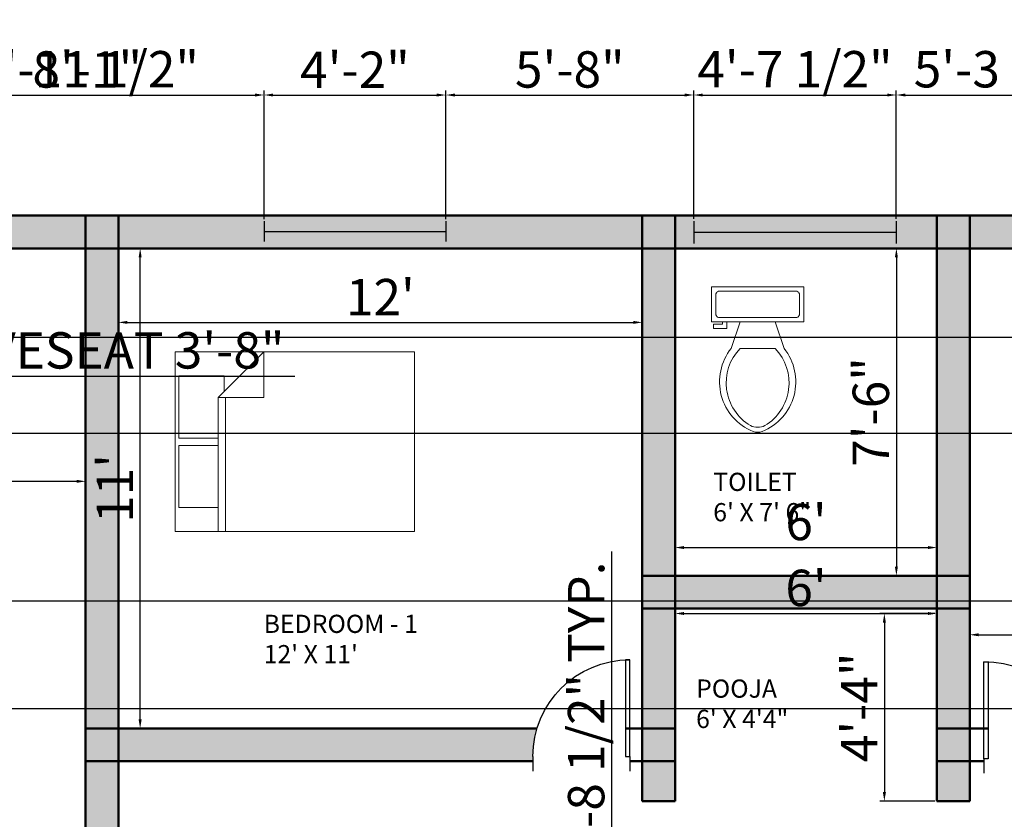
# Model space of a CAD drawing. Units: millimetres. Extents: x 2208 to 3043, y 878 to 1386.
# Tile 3 of 4: x 2479 to 2749, y 1166 to 1386. Entities that reach past the tile are written whole.
import ezdxf

# ---------------------------------------------------------------- set-up
doc = ezdxf.new("R2010")
doc.units = ezdxf.units.MM
for name, color, linetype, lineweight in [('A-ANNO-DIMS', 50, 'Continuous', 13), ('A-AREA-IDEN', 90, 'Continuous', 25), ('A-FLOR-FIXT', 140, 'Continuous', 18), ('A-WALL-PATT', 6, 'Continuous', 13), ('doors', 30, 'Continuous', 25), ('furniture', 140, 'Continuous', 18), ('walls', 200, 'Continuous', 50), ('windows', 10, 'Continuous', 25)]:
    doc.layers.add(name, color=color, linetype=linetype, lineweight=lineweight)
doc.styles.get("Standard").update_dxf_attribs({"font": 'arial.ttf'})
doc.dimstyles.new('ISO-25', dxfattribs={"dimtxt": 10, "dimasz": 2.5, "dimexe": 1.25, "dimexo": 0.625, "dimtad": 1, "dimdec": 0, "dimlunit": 3, "dimtxsty": 'Standard', "dimcen": 2.5, "dimadec": 0, "dimazin": 0, "dimtfac": 1, "dimtdec": 0, "dimtmove": 0, "dimatfit": 3, "dimfxl": 1, "dimarcsym": 0})

# ---------------------------------------------------------------- blocks, each defined once
blk = doc.blocks.new('*U2')
for p, q in [((0, 0), (0, -6)), ((40, 0), (40, -6))]:
    blk.add_line(p, q)
blk.add_lwpolyline([(0, 0), (0, 40), (1.75, 40), (1.75, 0)], close=True)
blk.add_arc((0, 0), 40, 0, 90)
blk = doc.blocks.new('*U4')
for p, q in [((0, 4), (0, 0)), ((36, 4), (36, 0)), ((0, 2), (36, 2))]:
    blk.add_line(p, q)
blk = doc.blocks.new('*U5')
for p, q in [((0, 4), (0, 0)), ((36, 4), (36, 0)), ((0, 2), (36, 2))]:
    blk.add_line(p, q)
blk = doc.blocks.new('Bed - Queen')
for p, q in [((0, -80.00003), (0, 0)), ((0, 0), (59.99999, 0)), ((59.99999, 0), (59.99999, -80.00003)), ((7.99999, -1.2), (28.79998, -1.2)), ((7.99999, -14.4), (7.99999, -1.2)), ((28.79998, -1.2), (28.79998, -14.4)), ((31.19999, -1.2), (51.99999, -1.2)), ((31.19999, -14.4), (31.19999, -1.2)), ((51.99999, -1.2), (51.99999, -16.4)), ((0, -14.4), (44.8, -14.4)), ((59.99999, -29.6), (44.8, -14.4)), ((44.8, -14.4), (44.8, -29.6)), ((51.99999, -16.4), (46.79936, -16.4)), ((44.8, -16.8), (0, -16.8)), ((44.8, -29.6), (59.99999, -29.6)), ((59.99999, -80.00003), (0, -80.00003))]:
    blk.add_line(p, q)
blk = doc.blocks.new('Toilet - top')
for p, q in [((9.5, -6), (9.5, -2)), ((-10, -8.5), (-8, -8.5)), ((-10, -9.5), (-10, -8.5)), ((-8, -8.5), (-8, -8)), ((-7, -8), (-7, -9.5)), ((-4, -8), (-6, -14)), ((4, -8), (6, -14)), ((-7, -9.5), (-10, -9.5)), ((4, -14), (-4, -14))]:
    blk.add_line(p, q)
blk.add_lwpolyline([(10.5, -8), (10.5, 0), (-10.5, 0), (-10.5, -8)], close=True)
for points in [[(-9.5, -2), (-9.5, -6)], [(8.5, -1), (-8.5, -1)], [(-8.5, -7), (8.5, -7)]]:
    blk.add_lwpolyline(points)
for centre, radius, start, end in [((-8.62, -1.88), 0.884, 81.8699, 188.1301), ((8.62, -1.88), 0.884, 351.8699, 98.1301), ((-8.62, -6.12), 0.884, 171.8699, 278.1301), ((8.62, -6.12), 0.884, 261.8699, 8.1301), ((3.52, -21.58), 12.17, 141.4691, 247.9714), ((4.2, -21.82), 11.33, 136.3677, 238.9468), ((-3.52, -21.58), 12.17, 292.0284, 38.5307), ((-4.2, -21.82), 11.33, 301.053, 43.6321), ((0, -27.88), 4, 245.7318, 294.2682), ((0, -29), 4, 254.8605, 285.1395)]:
    blk.add_arc(centre, radius, start, end)
blk = doc.blocks.new('*D13')
at = {"layer": 'A-ANNO-DIMS', "color": 0, "lineweight": -2, "transparency": 16777216}
for p, q in [((2505.98, 1310.26), (2505.98, 1301.83)), ((2649.98, 1310.26), (2649.98, 1301.83)), ((2508.48, 1303.08), (2647.48, 1303.08))]:
    blk.add_line(p, q, dxfattribs=at)
at = {"layer": 'A-ANNO-DIMS', "color": 0, "transparency": 16777216}
for points in [[(2508.48, 1303.5), (2508.48, 1302.67), (2505.98, 1303.08)], [(2647.48, 1303.5), (2647.48, 1302.67), (2649.98, 1303.08)]]:
    blk.add_solid(points, dxfattribs=at)
at = {"layer": 'Defpoints', "color": 0, "transparency": 16777216}
for p in [(2505.98, 1310.88), (2649.98, 1310.88), (2649.98, 1303.08)]:
    blk.add_point(p, dxfattribs=at)
at = {"layer": 'A-ANNO-DIMS', "color": 0, "transparency": 16777216, "insert": (2577.98, 1308.73), "char_height": 10, "attachment_point": 5}
blk.add_mtext("12'", dxfattribs=at)
blk = doc.blocks.new('*D14')
at = {"layer": 'A-ANNO-DIMS', "color": 0, "lineweight": -2, "transparency": 16777216}
for p, q in [((2514.03, 1323.44), (2510.71, 1323.44)), ((2511.96, 1193.94), (2511.96, 1320.94)), ((2514.03, 1191.44), (2510.71, 1191.44))]:
    blk.add_line(p, q, dxfattribs=at)
at = {"layer": 'A-ANNO-DIMS', "color": 0, "transparency": 16777216}
for points in [[(2511.54, 1320.94), (2512.37, 1320.94), (2511.96, 1323.44)], [(2511.54, 1193.94), (2512.37, 1193.94), (2511.96, 1191.44)]]:
    blk.add_solid(points, dxfattribs=at)
at = {"layer": 'Defpoints', "color": 0, "transparency": 16777216}
for p in [(2511.96, 1323.44), (2514.65, 1323.44), (2514.65, 1191.44)]:
    blk.add_point(p, dxfattribs=at)
at = {"layer": 'A-ANNO-DIMS', "color": 0, "transparency": 16777216, "insert": (2506.31, 1257.44), "char_height": 10, "attachment_point": 5, "rotation": 90}
blk.add_mtext("11'", dxfattribs=at)
blk = doc.blocks.new('*D15')
at = {"layer": 'A-ANNO-DIMS', "color": 0, "lineweight": -2, "transparency": 16777216}
for p, q in [((2352.98, 1251.32), (2352.98, 1260.64)), ((2355.48, 1259.39), (2494.48, 1259.39)), ((2496.98, 1251.32), (2496.98, 1260.64))]:
    blk.add_line(p, q, dxfattribs=at)
at = {"layer": 'A-ANNO-DIMS', "color": 0, "transparency": 16777216}
for points in [[(2355.48, 1259.81), (2355.48, 1258.97), (2352.98, 1259.39)], [(2494.48, 1259.81), (2494.48, 1258.97), (2496.98, 1259.39)]]:
    blk.add_solid(points, dxfattribs=at)
at = {"layer": 'Defpoints', "color": 0, "transparency": 16777216}
for p in [(2496.98, 1259.39), (2352.98, 1250.7), (2496.98, 1250.7)]:
    blk.add_point(p, dxfattribs=at)
at = {"layer": 'A-ANNO-DIMS', "color": 0, "transparency": 16777216, "insert": (2424.98, 1265.03), "char_height": 10, "attachment_point": 5}
blk.add_mtext("12'", dxfattribs=at)
blk = doc.blocks.new('*D17')
at = {"layer": 'A-ANNO-DIMS', "color": 0, "lineweight": -2, "transparency": 16777216}
for p, q in [((2658.98, 1251.31), (2658.98, 1239.93)), ((2730.98, 1251.31), (2730.98, 1239.93)), ((2661.48, 1241.18), (2728.48, 1241.18))]:
    blk.add_line(p, q, dxfattribs=at)
at = {"layer": 'A-ANNO-DIMS', "color": 0, "transparency": 16777216}
for points in [[(2661.48, 1241.6), (2661.48, 1240.77), (2658.98, 1241.18)], [(2728.48, 1241.6), (2728.48, 1240.77), (2730.98, 1241.18)]]:
    blk.add_solid(points, dxfattribs=at)
at = {"layer": 'Defpoints', "color": 0, "transparency": 16777216}
for p in [(2658.98, 1251.94), (2730.98, 1251.94), (2730.98, 1241.18)]:
    blk.add_point(p, dxfattribs=at)
at = {"layer": 'A-ANNO-DIMS', "color": 0, "transparency": 16777216, "insert": (2694.98, 1246.91), "char_height": 10, "attachment_point": 5}
blk.add_mtext("6'", dxfattribs=at)
blk = doc.blocks.new('*D18')
at = {"layer": 'A-ANNO-DIMS', "color": 0, "lineweight": -2, "transparency": 16777216}
for p, q in [((2709.59, 1323.44), (2721.07, 1323.44)), ((2719.82, 1320.94), (2719.82, 1235.94)), ((2709.59, 1233.44), (2721.07, 1233.44))]:
    blk.add_line(p, q, dxfattribs=at)
at = {"layer": 'A-ANNO-DIMS', "color": 0, "transparency": 16777216}
for points in [[(2719.41, 1320.94), (2720.24, 1320.94), (2719.82, 1323.44)], [(2719.41, 1235.94), (2720.24, 1235.94), (2719.82, 1233.44)]]:
    blk.add_solid(points, dxfattribs=at)
at = {"layer": 'Defpoints', "color": 0, "transparency": 16777216}
for p in [(2708.97, 1323.44), (2708.97, 1233.44), (2719.82, 1233.44)]:
    blk.add_point(p, dxfattribs=at)
at = {"layer": 'A-ANNO-DIMS', "color": 0, "transparency": 16777216, "insert": (2714.09, 1278.44), "char_height": 10, "attachment_point": 5, "rotation": 90}
blk.add_mtext('7\'-6"', dxfattribs=at)
blk = doc.blocks.new('*D19')
at = {"layer": 'A-ANNO-DIMS', "color": 0, "lineweight": -2, "transparency": 16777216}
for p, q in [((2739.98, 1223.81), (2739.98, 1215.95)), ((2913.98, 1223.81), (2913.98, 1215.95)), ((2742.48, 1217.2), (2911.48, 1217.2))]:
    blk.add_line(p, q, dxfattribs=at)
at = {"layer": 'A-ANNO-DIMS', "color": 0, "transparency": 16777216}
for points in [[(2742.48, 1217.62), (2742.48, 1216.78), (2739.98, 1217.2)], [(2911.48, 1217.62), (2911.48, 1216.78), (2913.98, 1217.2)]]:
    blk.add_solid(points, dxfattribs=at)
at = {"layer": 'Defpoints', "color": 0, "transparency": 16777216}
for p in [(2739.98, 1224.44), (2913.98, 1224.44), (2913.98, 1217.2)]:
    blk.add_point(p, dxfattribs=at)
at = {"layer": 'A-ANNO-DIMS', "color": 0, "transparency": 16777216, "insert": (2826.98, 1222.93), "char_height": 10, "attachment_point": 5}
blk.add_mtext('14\'-6"', dxfattribs=at)
blk = doc.blocks.new('*D31')
at = {"layer": 'A-ANNO-DIMS', "color": 0, "lineweight": -2, "transparency": 16777216}
for p, q in [((2658.98, 1216.36), (2658.98, 1224.31)), ((2730.98, 1216.36), (2730.98, 1224.31)), ((2661.48, 1223.06), (2728.48, 1223.06))]:
    blk.add_line(p, q, dxfattribs=at)
at = {"layer": 'A-ANNO-DIMS', "color": 0, "transparency": 16777216}
for points in [[(2661.48, 1223.47), (2661.48, 1222.64), (2658.98, 1223.06)], [(2728.48, 1223.47), (2728.48, 1222.64), (2730.98, 1223.06)]]:
    blk.add_solid(points, dxfattribs=at)
at = {"layer": 'Defpoints', "color": 0, "transparency": 16777216}
for p in [(2730.98, 1223.06), (2658.98, 1215.74), (2730.98, 1215.74)]:
    blk.add_point(p, dxfattribs=at)
at = {"layer": 'A-ANNO-DIMS', "color": 0, "transparency": 16777216, "insert": (2694.98, 1228.79), "char_height": 10, "attachment_point": 5}
blk.add_mtext("6'", dxfattribs=at)
blk = doc.blocks.new('*D32')
at = {"layer": 'A-ANNO-DIMS', "color": 0, "lineweight": -2, "transparency": 16777216}
for p, q in [((2730.36, 1223.06), (2715.27, 1223.06)), ((2716.52, 1220.56), (2716.52, 1173.94)), ((2730.36, 1171.44), (2715.27, 1171.44))]:
    blk.add_line(p, q, dxfattribs=at)
at = {"layer": 'A-ANNO-DIMS', "color": 0, "transparency": 16777216}
for points in [[(2716.11, 1220.56), (2716.94, 1220.56), (2716.52, 1223.06)], [(2716.11, 1173.94), (2716.94, 1173.94), (2716.52, 1171.44)]]:
    blk.add_solid(points, dxfattribs=at)
at = {"layer": 'Defpoints', "color": 0, "transparency": 16777216}
for p in [(2730.98, 1223.06), (2716.52, 1171.44), (2730.98, 1171.44)]:
    blk.add_point(p, dxfattribs=at)
at = {"layer": 'A-ANNO-DIMS', "color": 0, "transparency": 16777216, "insert": (2710.9, 1197.25), "char_height": 10, "attachment_point": 5, "rotation": 90}
blk.add_mtext('4\'-4"', dxfattribs=at)
blk = doc.blocks.new('*D34')
at = {"layer": 'A-ANNO-DIMS', "color": 0, "lineweight": -2, "transparency": 16777216}
for p, q in [((2641.64, 1104.85), (2641.64, 1240.09)), ((2642.27, 1104.85), (2640.39, 1104.85)), ((2641.64, 1099.01), (2641.64, 1102.35)), ((2642.27, 1096.51), (2640.39, 1096.51))]:
    blk.add_line(p, q, dxfattribs=at)
at = {"layer": 'A-ANNO-DIMS', "color": 0, "transparency": 16777216}
for points in [[(2641.22, 1102.35), (2642.06, 1102.35), (2641.64, 1104.85)], [(2641.22, 1099.01), (2642.06, 1099.01), (2641.64, 1096.51)]]:
    blk.add_solid(points, dxfattribs=at)
at = {"layer": 'Defpoints', "color": 0, "transparency": 16777216}
for p in [(2641.64, 1104.85), (2642.89, 1104.85), (2642.89, 1096.51)]:
    blk.add_point(p, dxfattribs=at)
at = {"layer": 'A-ANNO-DIMS', "color": 0, "transparency": 16777216, "insert": (2635.84, 1173.72), "char_height": 10, "attachment_point": 5, "rotation": 90}
blk.add_mtext('CHAIR 0\'-8 1/2" TYP.', dxfattribs=at)
blk = doc.blocks.new('*D44')
at = {"layer": 'A-ANNO-DIMS', "color": 0, "lineweight": -2, "transparency": 16777216}
for p, q in [((2402.99, 1294.26), (2402.99, 1287.04)), ((2446.98, 1294.26), (2446.98, 1287.04)), ((2405.49, 1288.29), (2444.48, 1288.29)), ((2446.98, 1288.29), (2554.51, 1288.29))]:
    blk.add_line(p, q, dxfattribs=at)
at = {"layer": 'A-ANNO-DIMS', "color": 0, "transparency": 16777216}
for points in [[(2405.49, 1288.7), (2405.49, 1287.87), (2402.99, 1288.29)], [(2444.48, 1288.7), (2444.48, 1287.87), (2446.98, 1288.29)]]:
    blk.add_solid(points, dxfattribs=at)
at = {"layer": 'Defpoints', "color": 0, "transparency": 16777216}
for p in [(2402.99, 1294.89), (2446.98, 1294.89), (2446.98, 1288.29)]:
    blk.add_point(p, dxfattribs=at)
at = {"layer": 'A-ANNO-DIMS', "color": 0, "transparency": 16777216, "insert": (2502, 1294.09), "char_height": 10, "attachment_point": 5}
blk.add_mtext('LOVESEAT 3\'-8"', dxfattribs=at)
blk = doc.blocks.new('*D47')
at = {"layer": 'A-ANNO-DIMS', "color": 0, "lineweight": -2, "transparency": 16777216}
for p, q in [((2343.36, 1332.44), (2309.12, 1332.44)), ((2310.37, 1329.94), (2310.37, 923.22)), ((2589.36, 920.72), (2309.12, 920.72))]:
    blk.add_line(p, q, dxfattribs=at)
at = {"layer": 'A-ANNO-DIMS', "color": 0, "transparency": 16777216}
for points in [[(2309.95, 1329.94), (2310.79, 1329.94), (2310.37, 1332.44)], [(2309.95, 923.22), (2310.79, 923.22), (2310.37, 920.72)]]:
    blk.add_solid(points, dxfattribs=at)
at = {"layer": 'Defpoints', "color": 0, "transparency": 16777216}
for p in [(2343.98, 1332.44), (2310.37, 920.72), (2589.98, 920.72)]:
    blk.add_point(p, dxfattribs=at)
at = {"layer": 'A-ANNO-DIMS', "color": 0, "transparency": 16777216, "insert": (2304.57, 1126.58), "char_height": 10, "attachment_point": 5, "rotation": 90}
blk.add_mtext('34\'-3 1/2"', dxfattribs=at)
blk = doc.blocks.new('*D51')
at = {"layer": 'A-ANNO-DIMS', "color": 0, "lineweight": -2, "transparency": 16777216}
for p, q in [((2344.15, 1299.03), (3035.56, 1299.03)), ((3034.31, 1296.53), (3034.31, 1275.14)), ((2344.61, 1272.64), (3035.56, 1272.64)), ((3034.31, 1272.64), (3034.31, 1218.83))]:
    blk.add_line(p, q, dxfattribs=at)
at = {"layer": 'A-ANNO-DIMS', "color": 0, "transparency": 16777216}
for points in [[(3033.9, 1296.53), (3034.73, 1296.53), (3034.31, 1299.03)], [(3033.9, 1275.14), (3034.73, 1275.14), (3034.31, 1272.64)]]:
    blk.add_solid(points, dxfattribs=at)
at = {"layer": 'Defpoints', "color": 0, "transparency": 16777216}
for p in [(2343.52, 1299.03), (2343.98, 1272.64), (3034.31, 1272.64)]:
    blk.add_point(p, dxfattribs=at)
at = {"layer": 'A-ANNO-DIMS', "color": 0, "transparency": 16777216, "insert": (3028.52, 1244.49), "char_height": 10, "attachment_point": 5, "rotation": 90}
blk.add_mtext('2\'-2 1/2"', dxfattribs=at)
blk = doc.blocks.new('*D55')
at = {"layer": 'A-ANNO-DIMS', "color": 0, "lineweight": -2, "transparency": 16777216}
for p, q in [((2448.81, 1332.56), (2448.81, 1366.84)), ((2546.02, 1331.5), (2546.02, 1366.84)), ((2451.31, 1365.59), (2543.52, 1365.59))]:
    blk.add_line(p, q, dxfattribs=at)
at = {"layer": 'A-ANNO-DIMS', "color": 0, "transparency": 16777216}
for points in [[(2451.31, 1366), (2451.31, 1365.17), (2448.81, 1365.59)], [(2543.52, 1366), (2543.52, 1365.17), (2546.02, 1365.59)]]:
    blk.add_solid(points, dxfattribs=at)
at = {"layer": 'Defpoints', "color": 0, "transparency": 16777216}
for p in [(2546.02, 1365.59), (2448.81, 1331.94), (2546.02, 1330.88)]:
    blk.add_point(p, dxfattribs=at)
at = {"layer": 'A-ANNO-DIMS', "color": 0, "transparency": 16777216, "insert": (2497.42, 1371.32), "char_height": 10, "attachment_point": 5}
blk.add_mtext('8\'-1"', dxfattribs=at)
blk = doc.blocks.new('*D56')
at = {"layer": 'A-ANNO-DIMS', "color": 0, "lineweight": -2, "transparency": 16777216}
for p, q in [((2546.02, 1331.5), (2546.02, 1366.84)), ((2595.97, 1331.5), (2595.97, 1366.84)), ((2548.52, 1365.59), (2593.47, 1365.59))]:
    blk.add_line(p, q, dxfattribs=at)
at = {"layer": 'A-ANNO-DIMS', "color": 0, "transparency": 16777216}
for points in [[(2548.52, 1366), (2548.52, 1365.17), (2546.02, 1365.59)], [(2593.47, 1366), (2593.47, 1365.17), (2595.97, 1365.59)]]:
    blk.add_solid(points, dxfattribs=at)
at = {"layer": 'Defpoints', "color": 0, "transparency": 16777216}
for p in [(2595.97, 1365.59), (2546.02, 1330.88), (2595.97, 1330.88)]:
    blk.add_point(p, dxfattribs=at)
at = {"layer": 'A-ANNO-DIMS', "color": 0, "transparency": 16777216, "insert": (2571, 1371.23), "char_height": 10, "attachment_point": 5}
blk.add_mtext('4\'-2"', dxfattribs=at)
blk = doc.blocks.new('*D57')
at = {"layer": 'A-ANNO-DIMS', "color": 0, "lineweight": -2, "transparency": 16777216}
for p, q in [((2595.97, 1331.5), (2595.97, 1366.84)), ((2664.12, 1331.57), (2664.12, 1366.84)), ((2598.47, 1365.59), (2661.62, 1365.59))]:
    blk.add_line(p, q, dxfattribs=at)
at = {"layer": 'A-ANNO-DIMS', "color": 0, "transparency": 16777216}
for points in [[(2598.47, 1366), (2598.47, 1365.17), (2595.97, 1365.59)], [(2661.62, 1366), (2661.62, 1365.17), (2664.12, 1365.59)]]:
    blk.add_solid(points, dxfattribs=at)
at = {"layer": 'Defpoints', "color": 0, "transparency": 16777216}
for p in [(2664.12, 1365.59), (2595.97, 1330.88), (2664.12, 1330.94)]:
    blk.add_point(p, dxfattribs=at)
at = {"layer": 'A-ANNO-DIMS', "color": 0, "transparency": 16777216, "insert": (2630.05, 1371.32), "char_height": 10, "attachment_point": 5}
blk.add_mtext('5\'-8"', dxfattribs=at)
blk = doc.blocks.new('*D58')
at = {"layer": 'A-ANNO-DIMS', "color": 0, "lineweight": -2, "transparency": 16777216}
for p, q in [((2664.12, 1331.57), (2664.12, 1366.84)), ((2719.8, 1331.57), (2719.8, 1366.84)), ((2666.62, 1365.59), (2717.3, 1365.59))]:
    blk.add_line(p, q, dxfattribs=at)
at = {"layer": 'A-ANNO-DIMS', "color": 0, "transparency": 16777216}
for points in [[(2666.62, 1366), (2666.62, 1365.17), (2664.12, 1365.59)], [(2717.3, 1366), (2717.3, 1365.17), (2719.8, 1365.59)]]:
    blk.add_solid(points, dxfattribs=at)
at = {"layer": 'Defpoints', "color": 0, "transparency": 16777216}
for p in [(2719.8, 1365.59), (2664.12, 1330.94), (2719.8, 1330.94)]:
    blk.add_point(p, dxfattribs=at)
at = {"layer": 'A-ANNO-DIMS', "color": 0, "transparency": 16777216, "insert": (2691.96, 1371.38), "char_height": 10, "attachment_point": 5}
blk.add_mtext('4\'-7 1/2"', dxfattribs=at)
blk = doc.blocks.new('*D59')
at = {"layer": 'A-ANNO-DIMS', "color": 0, "lineweight": -2, "transparency": 16777216}
for p, q in [((2719.8, 1331.57), (2719.8, 1366.84)), ((2783.08, 1330.66), (2783.08, 1366.84)), ((2722.3, 1365.59), (2780.58, 1365.59))]:
    blk.add_line(p, q, dxfattribs=at)
at = {"layer": 'A-ANNO-DIMS', "color": 0, "transparency": 16777216}
for points in [[(2722.3, 1366), (2722.3, 1365.17), (2719.8, 1365.59)], [(2780.58, 1366), (2780.58, 1365.17), (2783.08, 1365.59)]]:
    blk.add_solid(points, dxfattribs=at)
at = {"layer": 'Defpoints', "color": 0, "transparency": 16777216}
for p in [(2783.08, 1365.59), (2719.8, 1330.94), (2783.08, 1330.03)]:
    blk.add_point(p, dxfattribs=at)
at = {"layer": 'A-ANNO-DIMS', "color": 0, "transparency": 16777216, "insert": (2751.44, 1371.38), "char_height": 10, "attachment_point": 5}
blk.add_mtext('5\'-3 1/2"', dxfattribs=at)
blk = doc.blocks.new('*D63')
at = {"layer": 'A-ANNO-DIMS', "color": 0, "lineweight": -2, "transparency": 16777216}
for p, q in [((2406.08, 1227.17), (2406.08, 1366.84)), ((2465.35, 1227.17), (2465.35, 1366.84)), ((2408.58, 1365.59), (2462.85, 1365.59)), ((2465.35, 1365.59), (2527.15, 1365.59))]:
    blk.add_line(p, q, dxfattribs=at)
at = {"layer": 'A-ANNO-DIMS', "color": 0, "transparency": 16777216}
for points in [[(2408.58, 1366), (2408.58, 1365.17), (2406.08, 1365.59)], [(2462.85, 1366), (2462.85, 1365.17), (2465.35, 1365.59)]]:
    blk.add_solid(points, dxfattribs=at)
at = {"layer": 'Defpoints', "color": 0, "transparency": 16777216}
for p in [(2465.35, 1365.59), (2406.08, 1226.55), (2465.35, 1226.55)]:
    blk.add_point(p, dxfattribs=at)
at = {"layer": 'A-ANNO-DIMS', "color": 0, "transparency": 16777216, "insert": (2497.5, 1371.38), "char_height": 10, "attachment_point": 5}
blk.add_mtext('4\'-11 1/2"', dxfattribs=at)
blk = doc.blocks.new('*D64')
at = {"layer": 'A-ANNO-DIMS', "color": 0, "lineweight": -2, "transparency": 16777216}
for p, q in [((3034.31, 1226.55), (3034.31, 1280.35)), ((2465.97, 1226.55), (3035.56, 1226.55)), ((3034.31, 1199.41), (3034.31, 1224.05)), ((2465.97, 1196.91), (3035.56, 1196.91))]:
    blk.add_line(p, q, dxfattribs=at)
at = {"layer": 'A-ANNO-DIMS', "color": 0, "transparency": 16777216}
for points in [[(3033.9, 1224.05), (3034.73, 1224.05), (3034.31, 1226.55)], [(3033.9, 1199.41), (3034.73, 1199.41), (3034.31, 1196.91)]]:
    blk.add_solid(points, dxfattribs=at)
at = {"layer": 'Defpoints', "color": 0, "transparency": 16777216}
for p in [(2465.35, 1226.55), (3034.31, 1226.55), (2465.35, 1196.91)]:
    blk.add_point(p, dxfattribs=at)
at = {"layer": 'A-ANNO-DIMS', "color": 0, "transparency": 16777216, "insert": (3028.52, 1254.7), "char_height": 10, "attachment_point": 5, "rotation": 90}
blk.add_mtext('2\'-5 1/2"', dxfattribs=at)
blk = doc.blocks.new('*D66')
at = {"layer": 'A-ANNO-DIMS', "color": 0, "lineweight": -2, "transparency": 16777216}
for p, q in [((3034.31, 1140.35), (3034.31, 1201.74)), ((2674.33, 1140.35), (3035.56, 1140.35)), ((3034.31, 1095.26), (3034.31, 1137.85)), ((2673.86, 1092.76), (3035.56, 1092.76))]:
    blk.add_line(p, q, dxfattribs=at)
at = {"layer": 'A-ANNO-DIMS', "color": 0, "transparency": 16777216}
for points in [[(3033.9, 1137.85), (3034.73, 1137.85), (3034.31, 1140.35)], [(3033.9, 1095.26), (3034.73, 1095.26), (3034.31, 1092.76)]]:
    blk.add_solid(points, dxfattribs=at)
at = {"layer": 'Defpoints', "color": 0, "transparency": 16777216}
for p in [(2673.7, 1140.35), (3034.31, 1140.35), (2673.23, 1092.76)]:
    blk.add_point(p, dxfattribs=at)
at = {"layer": 'A-ANNO-DIMS', "color": 0, "transparency": 16777216, "insert": (3028.52, 1172.3), "char_height": 10, "attachment_point": 5, "rotation": 90}
blk.add_mtext('3\'-11 1/2"', dxfattribs=at)

msp = doc.modelspace()

# ---------------------------------------------------------------- hatches: boundary and pattern name
at = {"layer": 'A-WALL-PATT'}
h = msp.add_hatch(color=256, dxfattribs=at)
h.dxf.hatch_style = 1
h.paths.add_polyline_path([(2352.98, 1273, -0.051847), (2347.51, 1272.43), (2343.98, 1272.43), (2343.98, 1137.44), (2352.98, 1137.44)])
h.paths.add_polyline_path([(2352.98, 1323.44), (2343.98, 1323.44), (2343.98, 1299.03), (2347.51, 1299.03), (2352.98, 1299.03)])
h.paths.add_polyline_path([(2352.98, 1332.44), (2343.98, 1332.44), (2343.98, 1323.44), (2352.98, 1323.44)])
h.paths.add_polyline_path([(2496.98, 1332.44), (2352.98, 1332.44), (2352.98, 1323.44), (2496.98, 1323.44)])
h.paths.add_polyline_path([(2505.98, 1323.44), (2496.98, 1323.44), (2496.98, 1191.44), (2505.98, 1191.44)])
h.paths.add_polyline_path([(2505.98, 1332.44), (2496.98, 1332.44), (2496.98, 1323.44), (2505.98, 1323.44)])
h.paths.add_polyline_path([(2505.98, 1182.44), (2496.98, 1182.44), (2496.98, 1137.44), (2505.98, 1137.44)])
h.paths.add_polyline_path([(2505.98, 1191.44), (2496.98, 1191.44), (2496.98, 1182.44), (2505.98, 1182.44)])
h.paths.add_polyline_path([(2621.06, 1191.44), (2505.98, 1191.44), (2505.98, 1182.44), (2619.92, 1182.44), (2619.92, 1183.73, -0.073589)])
h.paths.add_polyline_path([(2496.98, 1137.44), (2352.98, 1137.44), (2352.98, 1128.44), (2496.98, 1128.44)])
h.paths.add_polyline_path([(2352.98, 1137.44), (2343.98, 1137.44), (2343.98, 1128.44), (2352.98, 1128.44)])
h.paths.add_polyline_path([(2352.98, 1128.44), (2343.98, 1128.44), (2343.98, 982.44), (2352.98, 982.44)])
h.paths.add_polyline_path([(2517.98, 1137.44), (2508.98, 1137.44), (2508.98, 1128.44), (2517.98, 1128.44)])
h.paths.add_polyline_path([(2505.98, 1137.44), (2496.98, 1137.44), (2496.98, 1128.44), (2505.98, 1128.44)])
h.paths.add_polyline_path([(2658.98, 1224.44), (2649.98, 1224.44), (2649.98, 1191.44), (2658.98, 1191.44)])
h.paths.add_polyline_path([(2658.98, 1323.44), (2649.98, 1323.44), (2649.98, 1233.44), (2658.98, 1233.44)])
h.paths.add_polyline_path([(2658.98, 1233.44), (2649.98, 1233.44), (2649.98, 1224.44), (2658.98, 1224.44)])
h.paths.add_polyline_path([(2730.98, 1233.44), (2658.98, 1233.44), (2658.98, 1224.44), (2730.98, 1224.44)])
h.paths.add_polyline_path([(2739.98, 1323.44), (2730.98, 1323.44), (2730.98, 1233.44), (2739.98, 1233.44)])
h.paths.add_polyline_path([(2739.98, 1224.44), (2730.98, 1224.44), (2730.98, 1191.44), (2739.98, 1191.44)])
h.paths.add_polyline_path([(2739.98, 1191.44), (2730.98, 1191.44), (2730.98, 1182.44), (2739.98, 1182.44)])
h.paths.add_polyline_path([(2739.98, 1182.44), (2730.98, 1182.44), (2730.98, 1171.44), (2739.98, 1171.44)])
h.paths.add_polyline_path([(2739.98, 972.44), (2730.98, 972.44), (2730.98, 929.72), (2602.15, 929.72), (2598.98, 929.72), (2598.98, 973.44), (2589.98, 973.44), (2589.98, 929.72), (2589.98, 920.72), (2730.98, 920.72), (2739.98, 920.72)])
h.paths.add_polyline_path([(2598.98, 1084.44), (2589.98, 1084.44), (2589.98, 982.44), (2598.98, 982.44)])
h.paths.add_polyline_path([(2598.98, 982.44), (2589.98, 982.44), (2589.98, 973.44), (2598.98, 973.44)])
h.paths.add_polyline_path([(2517.98, 973.44), (2508.98, 973.44), (2508.98, 944.53), (2517.98, 944.53)])
h.paths.add_polyline_path([(2517.98, 1044.76, -0.086498), (2508.98, 1043.19), (2508.98, 982.44), (2517.98, 982.44)])
h.paths.add_polyline_path([(2517.98, 982.44), (2508.98, 982.44), (2508.98, 973.44), (2517.98, 973.44)])
h.paths.add_polyline_path([(2352.98, 982.44), (2343.98, 982.44), (2343.98, 973.44), (2352.98, 973.44)])
h.paths.add_polyline_path([(2589.98, 1093.44), (2517.98, 1093.44), (2517.98, 1084.44), (2589.98, 1084.44)])
h.paths.add_polyline_path([(2517.98, 1093.44), (2508.98, 1093.44), (2508.98, 1084.44), (2517.98, 1084.44)])
h.paths.add_polyline_path([(2517.98, 1084.44), (2508.98, 1084.44), (2508.98, 1069.79), (2517.98, 1069.79)])
h.paths.add_polyline_path([(2517.98, 1100.83), (2517.21, 1100.83, -0.078775), (2508.98, 1102.14), (2508.98, 1093.44), (2517.98, 1093.44)])
h.paths.add_polyline_path([(2598.98, 1093.44), (2589.98, 1093.44), (2589.98, 1084.44), (2598.98, 1084.44)])
h.paths.add_polyline_path([(2802.98, 1122.44), (2730.98, 1122.44), (2730.98, 1113.44), (2802.98, 1113.44)])
h.paths.add_polyline_path([(2922.98, 1113.44), (2913.98, 1113.44), (2913.98, 981.44), (2922.98, 981.44)])
h.paths.add_polyline_path([(2856.98, 1069.77, -0.087206), (2847.98, 1067.81), (2847.98, 981.44), (2856.98, 981.44)])
h.paths.add_polyline_path([(2913.98, 981.44), (2856.98, 981.44), (2856.98, 972.44), (2913.98, 972.44)])
h.paths.add_polyline_path([(2856.98, 981.44), (2847.98, 981.44), (2847.98, 972.44), (2856.98, 972.44)])
h.paths.add_polyline_path([(2739.98, 995.72), (2739.98, 1004.72), (2730.98, 1004.72), (2730.98, 981.44), (2739.98, 981.44)])
h.paths.add_polyline_path([(2739.98, 981.44), (2730.98, 981.44), (2730.98, 972.44), (2739.98, 972.44)])
h.paths.add_polyline_path([(2922.98, 981.44), (2913.98, 981.44), (2913.98, 972.44), (2922.98, 972.44)])
h.paths.add_polyline_path([(3001.16, 1086.62), (2922.98, 1086.62), (2922.98, 1077.62), (3001.16, 1077.62)])
h.paths.add_polyline_path([(3001.16, 1191.44), (2922.98, 1191.44), (2922.98, 1182.44), (3001.16, 1182.44)])
h.paths.add_polyline_path([(2913.98, 1191.44), (2843.61, 1191.44), (2843.49, 1188.69, -0.05974), (2842.46, 1182.44), (2913.98, 1182.44)])
h.paths.add_polyline_path([(2922.98, 1191.44), (2913.98, 1191.44), (2913.98, 1182.44), (2922.98, 1182.44)])
h.paths.add_polyline_path([(2802.98, 1191.44), (2769.17, 1191.44, -0.079558), (2770.5, 1183.13), (2770.5, 1182.44), (2802.98, 1182.44)])
h.paths.add_polyline_path([(2811.98, 1191.44), (2802.98, 1191.44), (2802.98, 1182.44), (2811.98, 1182.44)])
h.paths.add_polyline_path([(2811.98, 1182.44), (2802.98, 1182.44), (2802.98, 1122.44), (2811.98, 1122.44)])
h.paths.add_polyline_path([(2811.98, 1122.44), (2802.98, 1122.44), (2802.98, 1113.44), (2811.98, 1113.44)])
h.paths.add_polyline_path([(2847.98, 1122.44), (2811.98, 1122.44), (2811.98, 1113.44), (2847.98, 1113.44)])
h.paths.add_polyline_path([(2856.98, 1122.44), (2847.98, 1122.44), (2847.98, 1113.44), (2856.98, 1113.44)])
h.paths.add_polyline_path([(2913.98, 1122.44), (2856.98, 1122.44), (2856.98, 1113.44), (2913.98, 1113.44)])
h.paths.add_polyline_path([(2922.98, 1122.44), (2913.98, 1122.44), (2913.98, 1113.44), (2922.98, 1113.44)])
h.paths.add_polyline_path([(2856.98, 1113.44), (2847.98, 1113.44), (2847.98, 1094.39), (2856.98, 1094.39)])
h.paths.add_polyline_path([(2922.98, 1323.44), (2913.98, 1323.44), (2913.98, 1191.44), (2922.98, 1191.44)])
h.paths.add_polyline_path([(2922.98, 1332.44), (2913.98, 1332.44), (2913.98, 1323.44), (2922.98, 1323.44)])
h.paths.add_polyline_path([(2913.98, 1332.44), (2739.98, 1332.44), (2739.98, 1323.44), (2913.98, 1323.44)])
h.paths.add_polyline_path([(2730.98, 1332.44), (2658.98, 1332.44), (2658.98, 1323.44), (2730.98, 1323.44)])
h.paths.add_polyline_path([(2649.98, 1332.44), (2505.98, 1332.44), (2505.98, 1323.44), (2649.98, 1323.44)])
h.paths.add_polyline_path([(2658.98, 1332.44), (2649.98, 1332.44), (2649.98, 1323.44), (2658.98, 1323.44)])
h.paths.add_polyline_path([(2739.98, 1332.44), (2730.98, 1332.44), (2730.98, 1323.44), (2739.98, 1323.44)])
h.paths.add_polyline_path([(2739.98, 1233.44), (2730.98, 1233.44), (2730.98, 1224.44), (2739.98, 1224.44)])
h.paths.add_polyline_path([(2658.98, 1191.44), (2649.98, 1191.44), (2649.98, 1182.44), (2658.98, 1182.44)])
h.paths.add_polyline_path([(2658.98, 1182.44), (2649.98, 1182.44), (2649.98, 1171.44), (2658.98, 1171.44)])
h.paths.add_polyline_path([(2508.98, 982.44), (2352.98, 982.44), (2352.98, 973.44), (2508.98, 973.44)])
h.paths.add_polyline_path([(2589.98, 982.44), (2517.98, 982.44), (2517.98, 973.44), (2589.98, 973.44)])
h.paths.add_polyline_path([(2730.98, 1004.72), (2598.98, 1004.72), (2598.98, 995.72), (2730.98, 995.72)])
h.paths.add_polyline_path([(2847.98, 981.44), (2739.98, 981.44), (2739.98, 972.44), (2847.98, 972.44)])

# ---------------------------------------------------------------- linework, layer by layer
at = {"layer": 'walls'}
for p, q in [((2343.98, 1332.44), (2922.98, 1332.44)), ((2496.98, 1332.44), (2496.98, 1128.44)), ((2505.98, 1332.44), (2505.98, 1128.44)), ((2649.98, 1332.44), (2649.98, 1171.44)), ((2658.98, 1332.44), (2658.98, 1171.44)), ((2730.98, 1332.44), (2730.98, 1171.44)), ((2739.98, 1332.44), (2739.98, 1171.44)), ((2343.98, 1323.44), (2922.98, 1323.44)), ((2649.98, 1233.44), (2739.98, 1233.44)), ((2649.98, 1224.44), (2739.98, 1224.44)), ((2496.98, 1191.44), (2621.06, 1191.44)), ((2496.98, 1191.44), (2621.06, 1191.44)), ((2645.36, 1191.44), (2658.98, 1191.44)), ((2645.36, 1191.44), (2658.98, 1191.44)), ((2730.98, 1191.44), (2745.06, 1191.44)), ((2496.98, 1182.44), (2619.92, 1182.44)), ((2496.98, 1182.44), (2619.92, 1182.44)), ((2646.53, 1182.44), (2658.98, 1182.44)), ((2646.53, 1182.44), (2658.98, 1182.44)), ((2730.98, 1182.44), (2743.9, 1182.44)), ((2649.98, 1171.44), (2658.98, 1171.44)), ((2730.98, 1171.44), (2739.98, 1171.44))]:
    msp.add_line(p, q, dxfattribs=at)

# ---------------------------------------------------------------- block references
at = {"layer": 'A-FLOR-FIXT', "xscale": 1.211687514206988, "yscale": 1.211687514206988, "zscale": 1.211687514206988}
msp.add_blockref('Toilet - top', (2681.69, 1312.89), dxfattribs=at)
at = {"layer": 'doors', "yscale": 0.6650461219051067, "zscale": 0.6650461219051067}
for p, xscale in [((2646.53, 1183.73), -0.6650461219051067), ((2743.9, 1183.13), 0.6650461219051067)]:
    msp.add_blockref('*U2', p, dxfattribs=dict(at, xscale=xscale))
at = {"layer": 'furniture', "xscale": 0.8230212393777605, "yscale": 0.8230212393777605, "zscale": 0.8230212393777605, "rotation": 90}
msp.add_blockref('Bed - Queen', (2521.57, 1245.58), dxfattribs=at)
at = {"layer": 'windows'}
for name, p, xscale, yscale, zscale in [('*U4', (2546.02, 1325.33), 1.38727767019332, 1.38727767019332, 1.38727767019332), ('*U5', (2664.12, 1324.75), 1.546623903893406, 1.546623903893406, 1.546623903893406)]:
    msp.add_blockref(name, p, dxfattribs=dict(at, xscale=xscale, yscale=yscale, zscale=zscale))

# ---------------------------------------------------------------- texts
at = {"layer": 'A-AREA-IDEN', "char_height": 5, "attachment_point": 1}
for s, width, insert in [('TOILET\\P6\' X 7\' 6"', 36.2721, (2669.48, 1261.74)), ("BEDROOM - 1 \\P12' X 11'", 73.1509, (2545.91, 1222.71)), ('POOJA\\P6\' X 4\'4"', 30.1995, (2664.77, 1204.91))]:
    msp.add_mtext_dynamic_manual_height_columns(s, width=width, gutter_width=12.5, heights=[0], dxfattribs=dict(at, insert=insert))

# ---------------------------------------------------------------- dimensions: what is measured, and where the dimension line sits
at = {"layer": 'A-ANNO-DIMS'}
for base, p1, p2, override, picture, middle in [((2465.35, 1365.59), (2406.08, 1226.55), (2465.35, 1226.55), {"dimdec": 1, "dimlfac": 1, "dimrnd": 0, "dimzin": 1, "dimdsep": 46, "dimlunit": 4, "dimfrac": 2}, '*D63', (2497.5, 1371.38)), ((2719.8, 1365.59), (2664.12, 1330.94), (2719.8, 1330.94), {"dimdec": 1, "dimlfac": 1, "dimrnd": 0, "dimzin": 1, "dimdsep": 46, "dimlunit": 4, "dimfrac": 2}, '*D58', (2691.96, 1371.38)), ((2783.08, 1365.59), (2719.8, 1330.94), (2783.08, 1330.03), {"dimdec": 1, "dimlfac": 1, "dimrnd": 0, "dimzin": 1, "dimdsep": 46, "dimlunit": 4, "dimfrac": 2}, '*D59', (2751.44, 1371.38)), ((2546.02, 1365.59), (2448.81, 1331.94), (2546.02, 1330.88), {"dimdec": 1, "dimlfac": 1, "dimrnd": 0, "dimzin": 1, "dimdsep": 46, "dimlunit": 4, "dimfrac": 2}, '*D55', (2497.42, 1371.32)), ((2595.9666, 1365.5855), (2546.0246, 1330.8762), (2595.9666, 1330.8762), {"dimdec": 1, "dimlfac": 1, "dimrnd": 0, "dimzin": 1, "dimdsep": 46, "dimlunit": 4, "dimfrac": 2}, '*D56', (2570.9956, 1371.231)), ((2664.1248, 1365.5855), (2595.9666, 1330.8762), (2664.1248, 1330.9413), {"dimdec": 1, "dimlfac": 1, "dimrnd": 0, "dimzin": 1, "dimdsep": 46, "dimlunit": 4, "dimfrac": 2}, '*D57', (2630.0457, 1371.3162)), ((2649.98, 1303.08), (2505.98, 1310.88), (2649.98, 1310.88), {"dimclrd": 0, "dimclre": 0, "dimclrt": 0}, '*D13', (2577.98, 1308.73)), ((2496.98, 1259.39), (2352.98, 1250.7), (2496.98, 1250.7), {"dimclrd": 0, "dimclre": 0, "dimclrt": 0}, '*D15', (2424.98, 1265.03)), ((2730.98, 1241.18), (2658.98, 1251.94), (2730.98, 1251.94), {"dimclrd": 0, "dimclre": 0, "dimclrt": 0}, '*D17', (2694.98, 1246.91)), ((2730.98, 1223.06), (2658.98, 1215.74), (2730.98, 1215.74), {"dimclrd": 0, "dimclre": 0, "dimclrt": 0}, '*D31', (2694.98, 1228.79)), ((2913.98, 1217.2), (2739.98, 1224.44), (2913.98, 1224.44), {"dimclrd": 0, "dimclre": 0, "dimclrt": 0}, '*D19', (2826.98, 1222.93))]:
    dim = msp.add_linear_dim(base=base, p1=p1, p2=p2, dimstyle='ISO-25', override=override, dxfattribs=at)
    dim.commit()
    dim.dimension.update_dxf_attribs({"geometry": picture, "text_midpoint": middle})
for base, p1, p2, override, picture, middle in [((2310.37, 920.72), (2343.98, 1332.44), (2589.98, 920.72), {"dimdec": 1, "dimlfac": 1, "dimrnd": 0, "dimzin": 1, "dimdsep": 46, "dimlunit": 4, "dimfrac": 2}, '*D47', (2304.57, 1126.58)), ((2511.96, 1323.44), (2514.65, 1191.44), (2514.65, 1323.44), {"dimclrd": 0, "dimclre": 0, "dimclrt": 0}, '*D14', (2506.31, 1257.44)), ((2719.82, 1233.44), (2708.97, 1323.44), (2708.97, 1233.44), {"dimclrd": 0, "dimclre": 0, "dimclrt": 0}, '*D18', (2714.09, 1278.44)), ((3034.31, 1272.64), (2343.52, 1299.03), (2343.98, 1272.64), {"dimdec": 1, "dimlfac": 1, "dimrnd": 0, "dimzin": 1, "dimdsep": 46, "dimlunit": 4, "dimfrac": 2}, '*D51', (3028.52, 1244.49)), ((3034.31, 1226.55), (2465.35, 1196.91), (2465.35, 1226.55), {"dimdec": 1, "dimlfac": 1, "dimrnd": 0, "dimzin": 1, "dimdsep": 46, "dimlunit": 4, "dimfrac": 2}, '*D64', (3028.52, 1254.7)), ((2716.52, 1171.44), (2730.98, 1223.06), (2730.98, 1171.44), {"dimclrd": 0, "dimclre": 0, "dimclrt": 0}, '*D32', (2710.9, 1197.25)), ((3034.31, 1140.35), (2673.23, 1092.76), (2673.7, 1140.35), {"dimdec": 1, "dimlfac": 1, "dimrnd": 0, "dimzin": 1, "dimdsep": 46, "dimlunit": 4, "dimfrac": 2}, '*D66', (3028.52, 1172.3))]:
    dim = msp.add_linear_dim(base=base, p1=p1, p2=p2, angle=90, dimstyle='ISO-25', override=override, dxfattribs=at)
    dim.commit()
    dim.dimension.update_dxf_attribs({"geometry": picture, "text_midpoint": middle})
dim = msp.add_linear_dim(base=(2446.98, 1288.29), p1=(2402.99, 1294.89), p2=(2446.98, 1294.89), text='LOVESEAT <>', dimstyle='ISO-25', override={"dimdec": 1, "dimlfac": 1, "dimrnd": 0, "dimzin": 1, "dimdsep": 46, "dimlunit": 4, "dimfrac": 2}, dxfattribs=at)
dim.commit()
dim.dimension.update_dxf_attribs({"geometry": '*D44', "text_midpoint": (2502, 1294.09)})
dim = msp.add_linear_dim(base=(2641.64, 1104.85), p1=(2642.89, 1096.51), p2=(2642.89, 1104.85), angle=90, text='CHAIR <> TYP.', dimstyle='ISO-25', override={"dimdec": 1, "dimlfac": 1, "dimrnd": 0, "dimzin": 1, "dimdsep": 46, "dimlunit": 4, "dimfrac": 2}, dxfattribs=at)
dim.commit()
dim.dimension.update_dxf_attribs({"geometry": '*D34', "text_midpoint": (2635.84, 1173.72)})

doc.saveas('drawing.dxf')
